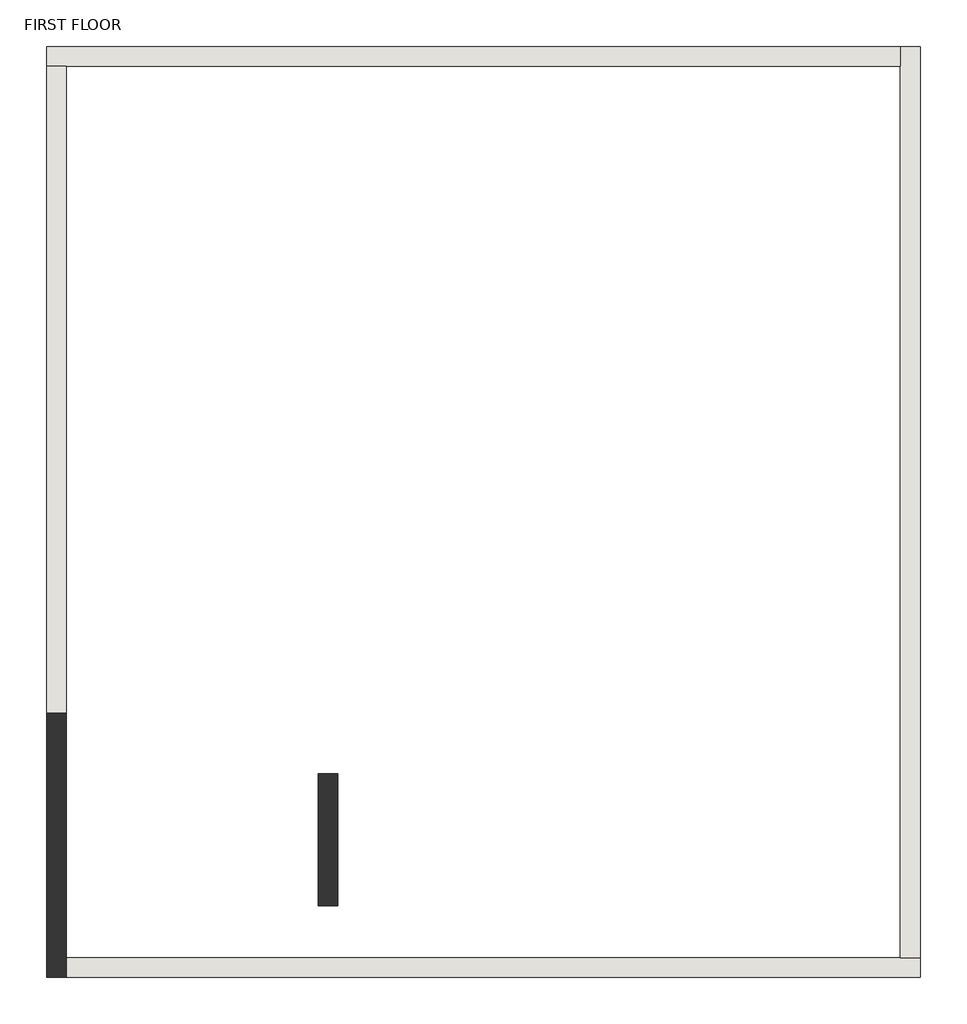
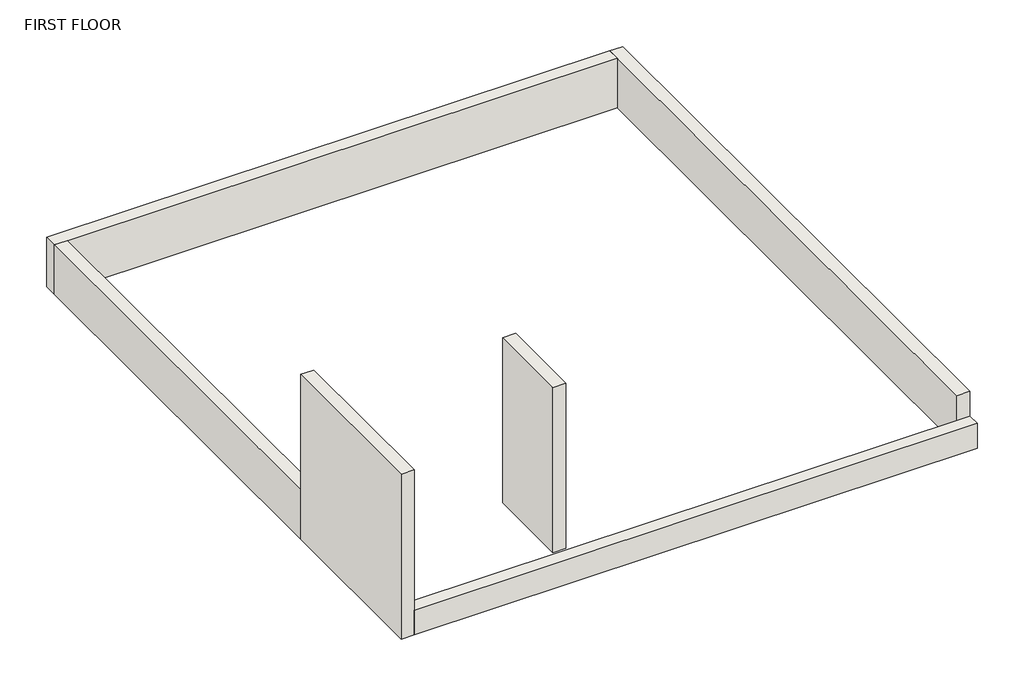
# One storey: 6 walls.
"""IFC4 building model written with IfcOpenShell, lengths in millimetres."""

from ifc_helpers import new_model, si_unit, frame, origin, place, context, project, spatial, polyline, outline, extrude, faceted_brep, element, save

model = new_model("IFC4")

# Units and contexts
model_context = context("Model", 3, world=origin())
ifc_project = project(units=[si_unit("LENGTHUNIT", "METRE", prefix="MILLI")], contexts=[model_context])

# Site, building, storey
site = spatial("IfcSite", under=ifc_project)
building = spatial("IfcBuilding", under=site)
storey = spatial("IfcBuildingStorey", under=building, Name="FIRST FLOOR", Elevation=6705.6)

# Walls
placement = place(None, origin())
element("IfcWall", 1, ObjectType="wall 9\"", at=placement, inside=storey, context=model_context, shape_type="Brep", body=[
    faceted_brep([(-9380.7179063, 69.3888401, 6705.6), (-9380.7179063, 297.9888401, 6705.6), (-9380.7179063, 3117.3888401, 6705.6), (-9380.7179063, 3117.3888401, 7620.0), (-9380.7179063, 3117.3888401, 9753.6), (-9380.7179063, 69.3888401, 9753.6), (-9380.7179063, 69.3888401, 7162.8), (-9609.3179063, 69.3888401, 6705.6), (-9609.3179063, 69.3888401, 9753.6), (-9609.3179063, 3117.3888401, 9753.6), (-9609.3179063, 3117.3888401, 7620.0), (-9609.3179063, 3117.3888401, 6705.6)], [[[0, 1, 2, 3, 4, 5, 6]], [[7, 8, 9, 10, 11]], [[2, 1, 0, 7, 11]], [[4, 3, 2, 11, 10, 9]], [[5, 4, 9, 8]], [[0, 6, 5, 8, 7]]]),
])
element("IfcWall", 2, ObjectType="wall 9\"", at=placement, inside=storey, context=model_context, shape_type="Brep", body=[
    faceted_brep([(-9380.7179063, 69.3888401, 6705.6), (474.4820937, 69.3888401, 6705.6), (474.4820937, 69.3888401, 7162.8), (-9380.7179063, 69.3888401, 7162.8), (-9380.7179063, 297.9888401, 6705.6), (-9380.7179063, 297.9888401, 7162.8), (474.4820937, 297.9888401, 7162.8), (474.4820937, 297.9888401, 6705.6), (245.8820937, 297.9888401, 6705.6)], [[[0, 1, 2, 3]], [[4, 5, 6, 7, 8]], [[1, 0, 4, 8, 7]], [[3, 2, 6, 5]], [[0, 3, 5, 4]], [[2, 1, 7, 6]]]),
])
element("IfcWall", 3, ObjectType="wall 9\"", at=placement, inside=storey, context=model_context, shape_type="Brep", body=[
    faceted_brep([(474.4820937, 297.9888401, 6705.6), (474.4820937, 10813.5888401, 6705.6), (474.4820937, 10813.5888401, 7620.0), (474.4820937, 297.9888401, 7620.0), (474.4820937, 297.9888401, 7162.8), (245.8820937, 297.9888401, 6705.6), (245.8820937, 297.9888401, 7620.0), (245.8820937, 10584.9888401, 7620.0), (245.8820937, 10813.5888401, 7620.0), (245.8820937, 10813.5888401, 6705.6), (245.8820937, 10584.9888401, 6705.6)], [[[0, 1, 2, 3, 4]], [[5, 6, 7, 8, 9, 10]], [[1, 0, 5, 10, 9]], [[3, 2, 8, 7, 6]], [[0, 4, 3, 6, 5]], [[2, 1, 9, 8]]]),
])
element("IfcWall", 4, ObjectType="wall 9\"", at=placement, inside=storey, context=model_context, shape_type="Brep", body=[
    faceted_brep([(245.8820937, 10813.5888401, 6705.6), (-9609.3179063, 10813.5888401, 6705.6), (-9609.3179063, 10813.5888401, 7620.0), (245.8820937, 10813.5888401, 7620.0), (245.8820937, 10584.9888401, 6705.6), (245.8820937, 10584.9888401, 7620.0), (-9380.7179063, 10584.9888401, 7620.0), (-9609.3179063, 10584.9888401, 7620.0), (-9609.3179063, 10584.9888401, 6705.6), (-9380.7179063, 10584.9888401, 6705.6)], [[[0, 1, 2, 3]], [[4, 5, 6, 7, 8, 9]], [[1, 0, 4, 9, 8]], [[3, 2, 7, 6, 5]], [[0, 3, 5, 4]], [[2, 1, 8, 7]]]),
])
element("IfcWall", 5, ObjectType="wall 9\"", at=placement, inside=storey, context=model_context, shape_type="SweptSolid", body=[
    extrude(outline(polyline([(-9609.3179063, 3117.3888401), (-9609.3179063, 10584.9888401), (-9380.7179063, 10584.9888401), (-9380.7179063, 3117.3888401), (-9609.3179063, 3117.3888401)])), frame((0.0, 0.0, 6705.6), z_axis=(0.0, 0.0, 1.0), x_axis=(1.0, 0.0, 0.0)), (0.0, 0.0, 1.0), 914.4),
])
element("IfcWall", 6, ObjectType="wall 9\"", at=placement, inside=storey, context=model_context, shape_type="SweptSolid", body=[
    extrude(outline(polyline([(-6247.3892099, 2423.1698373), (-6247.3892099, 899.1698373), (-6475.9892099, 899.1698373), (-6475.9892099, 2423.1698373), (-6247.3892099, 2423.1698373)])), frame((0.0, 0.0, 6705.6), z_axis=(0.0, 0.0, 1.0), x_axis=(1.0, 0.0, 0.0)), (0.0, 0.0, 1.0), 3048.0),
])

save(model, "model.ifc")

# Revit data of these elements
# Type "wall 9\""
#   Assembly Code = "B2010"
#   Layers, outside or top first: 0' - 9" no material (function 1)
# Element 1 (IfcWall, "wall 9\"")
#   Top Offset = 0' - 0"
#   Base Offset = 0' - 0"
#   Unconnected Height = 10' - 0"
#   wall height = 10' - 0"
#   Phase Created = New Construction
#   Base Constraint = FIRST FLOOR
#   Materials on its faces: "Default Wall"
# Element 2 (IfcWall, "wall 9\"")
#   Top Offset = 0' - 0"
#   Base Offset = 0' - 0"
#   wall height = 1' - 6"
#   Phase Created = New Construction
#   Base Constraint = FIRST FLOOR
#   Top Constraint = Level 4
#   Materials on its faces: "Default Wall"
# Elements 3, 4, 5 (IfcWall, "wall 9\"")
#   Top Offset = 0' - 0"
#   Base Offset = 0' - 0"
#   wall height = 3' - 0"
#   Phase Created = New Construction
#   Base Constraint = FIRST FLOOR
#   Top Constraint = Level 5
#   Materials on its faces: "Default Wall"
# Element 6 (IfcWall, "wall 9\"")
#   Top Offset = 0' - 0"
#   Base Offset = 0' - 0"
#   wall height = 10' - 0"
#   Phase Created = New Construction
#   Base Constraint = FIRST FLOOR
#   Top Constraint = TOP
#   Materials on its faces: "Default Wall"
# Materials
#   "Default Wall": colour RGB 128 128 128, transparency 0, Cost = 0
